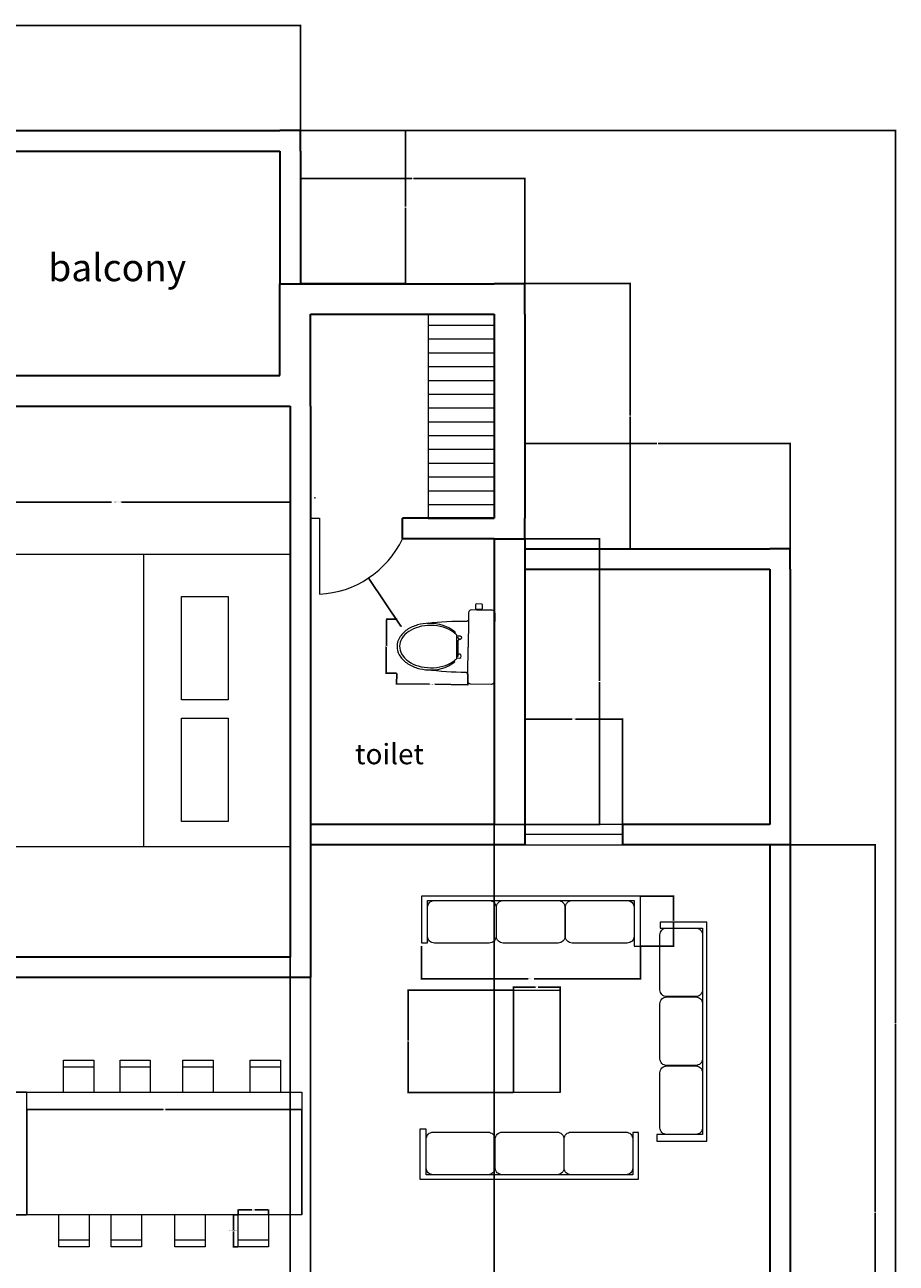
# Model space of a CAD drawing. Units: inches. Extents: x 177 to 785, y -381 to 206.
# Tile 5 of 5: x 529 to 785, y -158 to 206. Entities that reach past the tile are written whole.
import ezdxf

# ---------------------------------------------------------------- set-up
doc = ezdxf.new("R2010")
doc.units = ezdxf.units.IN
doc.header["$MEASUREMENT"] = 0
for name, color, linetype, lineweight in [('A-ANNO-DIMS', 2, 'Continuous', 18), ('A-AREA-IDEN', 7, 'Continuous', 20), ('A-DOOR', 4, 'Continuous', 18), ('A-FLOR-CASE', 9, 'Continuous', 20), ('A-FLOR-CASE-PATT', 9, 'Continuous', 13), ('A-FLOR-FIXT', 8, 'Continuous', 18), ('A-FURN', 2, 'Continuous', 18), ('A-GLAZ', 4, 'Continuous', 18), ('A-WALL', 7, 'Continuous', 35), ('WC-Detail_dwgmodels.com', 9, 'Continuous', 13), ('WC-Outline_dwgmodels.com', 8, 'Continuous', 18)]:
    doc.layers.add(name, color=color, linetype=linetype, lineweight=lineweight)
doc.styles.get("Standard").update_dxf_attribs({"font": 'arial.ttf'})
doc.dimstyles.get("Standard").update_dxf_attribs({"dimtxt": 0.18, "dimasz": 0.18, "dimexe": 0.18, "dimexo": 0.0625, "dimgap": 0.09, "dimtad": 0, "dimtih": 1, "dimtoh": 1, "dimdec": 4, "dimzin": 0, "dimdsep": 46, "dimtxsty": 'Standard', "dimcen": 0.09, "dimadec": 0, "dimazin": 0, "dimtfac": 1, "dimtdec": 4, "dimtofl": 0, "dimtmove": 0, "dimatfit": 3, "dimfxl": 1, "dimtolj": 1, "dimtzin": 0, "dimarcsym": 0})

# ---------------------------------------------------------------- blocks, each defined once
blk = doc.blocks.new('BED-DOUBLE')
blk.add_line((58.96, 86.04), (58.96, 0))
for points in [[(0, 86.04), (102.05, 86.04), (102.05, 0), (0, 0)], [(70.1, 73.56), (83.84, 73.56), (83.84, 43.2), (70.1, 43.2)], [(70.1, 37.79), (83.84, 37.79), (83.84, 7.42), (70.1, 7.42)]]:
    blk.add_lwpolyline(points, close=True)
blk = doc.blocks.new('SOFA-3-SEAT')
for p, q in [((64.37, 14.65), (0, 14.65)), ((0, 14.65), (0, 0.95)), ((64.37, 0), (64.37, 14.65)), ((1.74, 11.38), (1.74, 13.38)), ((1.74, 13.38), (62.42, 13.38)), ((62.42, 13.38), (62.42, 0)), ((0, 0.95), (1.74, 0.95)), ((1.74, 0.95), (1.74, 2.86)), ((62.42, 0), (64.37, 0))]:
    blk.add_line(p, q)
for points in [[(3.74, 13.38), (19.89, 13.38, -0.414214), (21.89, 11.38), (21.89, 2.86, -0.414214), (19.89, 0.86), (3.74, 0.86, -0.414214), (1.74, 2.86), (1.74, 11.38, -0.414214)], [(23.98, 13.38), (40.13, 13.38, -0.414214), (42.13, 11.38), (42.13, 2.86, -0.414214), (40.13, 0.86), (23.98, 0.86, -0.414214), (21.98, 2.86), (21.98, 11.38, -0.414214)], [(44.27, 13.38), (60.42, 13.38, -0.414214), (62.42, 11.38), (62.42, 2.86, -0.414214), (60.42, 0.86), (44.27, 0.86, -0.414214), (42.27, 2.86), (42.27, 11.38, -0.414214)]]:
    blk.add_lwpolyline(points, format="xyb", close=True)
blk = doc.blocks.new('CHAIR-DINING')
for p, q in [((0, 9.42), (8.88, 9.42)), ((0, 7.42), (0, 9.42)), ((0, 0), (0, 7.42)), ((0, 7.42), (8.88, 7.42)), ((8.88, 9.42), (8.88, 7.42)), ((8.88, 7.42), (8.88, 0))]:
    blk.add_line(p, q)
blk = doc.blocks.new('WC-PAN-AND-SEAT')
for points in [[(0, 20.91, -0.279901), (0.43, 20.4, 0.030761), (1.12, 8.8, 16.522544)], [(15.88, 20.91, 0.279901), (15.45, 20.4, -0.030761), (14.76, 8.8, -16.522544)], [(1.08, 9.29, -0.186192), (3.55, 17.08), (3.86, 16.84)], [(1.72, 9.92, 0.068564), (2.22, 6.28, 0.080689), (3.54, 3.43, 0.107047), (5.7, 1.38, 0.137952), (7.94, 0.75, 0.137952), (10.18, 1.38, 0.107047), (12.34, 3.43, 0.080689), (13.66, 6.28, 0.068564), (14.16, 9.92, 0.068564), (13.66, 13.57, 0.080689), (12.34, 16.41, 0.049741), (11.45, 17.48, 0.137952)], [(4.44, 17.48, 0.049741), (3.54, 16.41, 0.080689), (2.22, 13.57, 0.068564), (1.72, 9.92, 0.068564)], [(14.76, 8.8, 0.197511), (12.33, 17.08), (12.02, 16.84)], [(1.07, 9.29, 0.059006), (1.61, 5.99, 0.081908), (3.07, 2.91, 0.106902), (5.45, 0.69, 0.135271), (7.94, 0, 0.135271)], [(1.12, 8.8, -0.010918), (1.08, 9.29)], [(7.94, 0, 0.135271), (10.44, 0.69, 0.106902), (12.81, 2.91, 0.081908), (14.28, 5.99, 0.059006), (14.82, 9.29, 0.070136)]]:
    blk.add_lwpolyline(points, format="xyb")
blk.add_lwpolyline([(4.44, 17.48), (11.45, 17.48)])
blk = doc.blocks.new('*D9')
at = {"layer": 'A-ANNO-DIMS', "color": 0, "lineweight": -2, "transparency": 16777216}
for p, q in [((592, -143.94), (590.47, -143.94)), ((590.65, -144.12), (590.65, -148.47)), ((590.65, -153.18), (590.65, -148.83)), ((592, -153.36), (590.47, -153.36))]:
    blk.add_line(p, q, dxfattribs=at)
at = {"layer": 'A-ANNO-DIMS', "color": 0, "transparency": 16777216}
for points in [[(590.62, -144.12), (590.68, -144.12), (590.65, -143.94)], [(590.62, -153.18), (590.68, -153.18), (590.65, -153.36)]]:
    blk.add_solid(points, dxfattribs=at)
at = {"layer": 'Defpoints', "color": 0, "transparency": 16777216}
for p in [(592.07, -143.94), (590.65, -153.36), (592.07, -153.36)]:
    blk.add_point(p, dxfattribs=at)
at = {"layer": 'A-ANNO-DIMS', "color": 0, "transparency": 16777216, "insert": (590.65, -148.65), "char_height": 0.18, "attachment_point": 5}
blk.add_mtext('\\A1;DINING CHAIR 9 TYP.', dxfattribs=at)
blk = doc.blocks.new('*D10')
at = {"layer": 'A-ANNO-DIMS', "color": 0, "lineweight": -2, "transparency": 16777216}
for p, q in [((592.07, -143.88), (592.07, -142.34)), ((592.25, -142.52), (596.05, -142.52)), ((600.77, -142.52), (596.96, -142.52)), ((600.95, -143.88), (600.95, -142.34))]:
    blk.add_line(p, q, dxfattribs=at)
at = {"layer": 'A-ANNO-DIMS', "color": 0, "transparency": 16777216}
for points in [[(592.25, -142.49), (592.25, -142.55), (592.07, -142.52)], [(600.77, -142.49), (600.77, -142.55), (600.95, -142.52)]]:
    blk.add_solid(points, dxfattribs=at)
at = {"layer": 'Defpoints', "color": 0, "transparency": 16777216}
for p in [(592.07, -142.52), (592.07, -143.94), (600.95, -143.94)]:
    blk.add_point(p, dxfattribs=at)
at = {"layer": 'A-ANNO-DIMS', "color": 0, "transparency": 16777216, "insert": (596.51, -142.52), "char_height": 0.18, "attachment_point": 5}
blk.add_mtext('\\A1;9 TYP.', dxfattribs=at)
blk = doc.blocks.new('*D13')
at = {"layer": 'A-ANNO-DIMS', "color": 0, "lineweight": -2, "transparency": 16777216}
for p, q in [((505.28, 50.4), (505.28, 65.83)), ((505.46, 65.65), (554.86, 65.65)), ((607.15, 65.65), (557.74, 65.65)), ((607.33, 50.4), (607.33, 65.83))]:
    blk.add_line(p, q, dxfattribs=at)
at = {"layer": 'A-ANNO-DIMS', "color": 0, "transparency": 16777216}
for points in [[(505.46, 65.68), (505.46, 65.62), (505.28, 65.65)], [(607.15, 65.68), (607.15, 65.62), (607.33, 65.65)]]:
    blk.add_solid(points, dxfattribs=at)
at = {"layer": 'Defpoints', "color": 0, "transparency": 16777216}
for p in [(607.33, 65.65), (505.28, 50.34), (607.33, 50.34)]:
    blk.add_point(p, dxfattribs=at)
at = {"layer": 'A-ANNO-DIMS', "color": 0, "transparency": 16777216, "insert": (556.3, 65.65), "char_height": 0.18, "attachment_point": 5}
blk.add_mtext('\\A1;DOUBLE BED 102 TYP.', dxfattribs=at)
blk = doc.blocks.new('*D15')
at = {"layer": 'A-ANNO-DIMS', "color": 0, "lineweight": -2, "transparency": 16777216}
for p, q in [((645.99, -64.97), (645.99, -74.74)), ((710.36, -64.97), (710.36, -74.74)), ((646.17, -74.56), (677.27, -74.56)), ((710.18, -74.56), (679.08, -74.56))]:
    blk.add_line(p, q, dxfattribs=at)
at = {"layer": 'A-ANNO-DIMS', "color": 0, "transparency": 16777216}
for points in [[(646.17, -74.53), (646.17, -74.59), (645.99, -74.56)], [(710.18, -74.53), (710.18, -74.59), (710.36, -74.56)]]:
    blk.add_solid(points, dxfattribs=at)
at = {"layer": 'Defpoints', "color": 0, "transparency": 16777216}
for p in [(645.99, -64.91), (710.36, -64.91), (710.36, -74.56)]:
    blk.add_point(p, dxfattribs=at)
at = {"layer": 'A-ANNO-DIMS', "color": 0, "transparency": 16777216, "insert": (678.17, -74.56), "char_height": 0.18, "attachment_point": 5}
blk.add_mtext('\\A1;SOFA 64 TYP.', dxfattribs=at)
blk = doc.blocks.new('*D16')
at = {"layer": 'A-ANNO-DIMS', "color": 0, "lineweight": -2, "transparency": 16777216}
for p, q in [((710.42, -50.26), (720.19, -50.26)), ((720.01, -50.44), (720.01, -57.4)), ((720.01, -64.73), (720.01, -57.77)), ((710.42, -64.91), (720.19, -64.91))]:
    blk.add_line(p, q, dxfattribs=at)
at = {"layer": 'A-ANNO-DIMS', "color": 0, "transparency": 16777216}
for points in [[(719.98, -50.44), (720.04, -50.44), (720.01, -50.26)], [(719.98, -64.73), (720.04, -64.73), (720.01, -64.91)]]:
    blk.add_solid(points, dxfattribs=at)
at = {"layer": 'Defpoints', "color": 0, "transparency": 16777216}
for p in [(710.36, -50.26), (720.01, -50.26), (710.36, -64.91)]:
    blk.add_point(p, dxfattribs=at)
at = {"layer": 'A-ANNO-DIMS', "color": 0, "transparency": 16777216, "insert": (720.01, -57.58), "char_height": 0.18, "attachment_point": 5}
blk.add_mtext('\\A1;15 TYP.', dxfattribs=at)
blk = doc.blocks.new('*D17')
at = {"layer": 'A-ANNO-DIMS', "color": 0, "lineweight": -2, "transparency": 16777216}
for p, q in [((638.65, 15.24), (638.62, 11.99)), ((659.56, 15.01), (659.52, 11.76)), ((638.8, 12.17), (648.29, 12.06)), ((659.34, 11.94), (649.85, 12.05))]:
    blk.add_line(p, q, dxfattribs=at)
at = {"layer": 'A-ANNO-DIMS', "color": 0, "transparency": 16777216}
for points in [[(638.8, 12.2), (638.8, 12.14), (638.62, 12.17)], [(659.34, 11.97), (659.34, 11.91), (659.52, 11.94)]]:
    blk.add_solid(points, dxfattribs=at)
at = {"layer": 'Defpoints', "color": 0, "transparency": 16777216}
for p in [(638.65, 15.31), (659.56, 15.07), (659.52, 11.94)]:
    blk.add_point(p, dxfattribs=at)
at = {"layer": 'A-ANNO-DIMS', "color": 0, "transparency": 16777216, "insert": (649.07, 12.05), "char_height": 0.18, "attachment_point": 5}
blk.add_mtext('\\A1;WC 21 TYP.', dxfattribs=at)
blk = doc.blocks.new('*D18')
at = {"layer": 'A-ANNO-DIMS', "color": 0, "lineweight": -2, "transparency": 16777216}
for p, q in [((638.77, 31.19), (635.51, 31.22)), ((635.69, 31.04), (635.61, 23.46)), ((635.52, 15.52), (635.6, 23.1)), ((638.59, 15.31), (635.34, 15.34))]:
    blk.add_line(p, q, dxfattribs=at)
at = {"layer": 'A-ANNO-DIMS', "color": 0, "transparency": 16777216}
for points in [[(635.66, 31.04), (635.72, 31.04), (635.69, 31.22)], [(635.49, 15.52), (635.55, 15.52), (635.52, 15.34)]]:
    blk.add_solid(points, dxfattribs=at)
at = {"layer": 'Defpoints', "color": 0, "transparency": 16777216}
for p in [(638.83, 31.19), (635.52, 15.34), (638.65, 15.31)]:
    blk.add_point(p, dxfattribs=at)
at = {"layer": 'A-ANNO-DIMS', "color": 0, "transparency": 16777216, "insert": (635.61, 23.28), "char_height": 0.18, "attachment_point": 5}
blk.add_mtext('\\A1;16 TYP.', dxfattribs=at)
blk = doc.blocks.new('*D24')
at = {"layer": 'A-ANNO-DIMS', "color": 0, "lineweight": -2, "transparency": 16777216}
for p, q in [((610.39, 174.86), (785.46, 174.86)), ((785.28, 174.68), (785.28, -87.46)), ((785.28, -349.96), (785.28, -87.82)), ((537.67, -350.14), (785.46, -350.14))]:
    blk.add_line(p, q, dxfattribs=at)
at = {"layer": 'A-ANNO-DIMS', "color": 0, "transparency": 16777216}
for points in [[(785.25, 174.68), (785.31, 174.68), (785.28, 174.86)], [(785.25, -349.96), (785.31, -349.96), (785.28, -350.14)]]:
    blk.add_solid(points, dxfattribs=at)
at = {"layer": 'Defpoints', "color": 0, "transparency": 16777216}
for p in [(610.33, 174.86), (537.61, -350.14), (785.28, -350.14)]:
    blk.add_point(p, dxfattribs=at)
at = {"layer": 'A-ANNO-DIMS', "color": 0, "transparency": 16777216, "insert": (785.28, -87.64), "char_height": 0.18, "attachment_point": 5}
blk.add_mtext('\\A1;525', dxfattribs=at)
blk = doc.blocks.new('*D27')
at = {"layer": 'A-ANNO-DIMS', "color": 0, "lineweight": -2, "transparency": 16777216}
for p, q in [((355.33, 174.92), (355.33, 205.99)), ((355.51, 205.81), (482.54, 205.81)), ((610.15, 205.81), (483.12, 205.81)), ((610.33, 174.92), (610.33, 205.99))]:
    blk.add_line(p, q, dxfattribs=at)
at = {"layer": 'A-ANNO-DIMS', "color": 0, "transparency": 16777216}
for points in [[(355.51, 205.84), (355.51, 205.78), (355.33, 205.81)], [(610.15, 205.84), (610.15, 205.78), (610.33, 205.81)]]:
    blk.add_solid(points, dxfattribs=at)
at = {"layer": 'Defpoints', "color": 0, "transparency": 16777216}
for p in [(610.33, 205.81), (355.33, 174.86), (610.33, 174.86)]:
    blk.add_point(p, dxfattribs=at)
at = {"layer": 'A-ANNO-DIMS', "color": 0, "transparency": 16777216, "insert": (482.83, 205.81), "char_height": 0.18, "attachment_point": 5}
blk.add_mtext('\\A1;255', dxfattribs=at)
blk = doc.blocks.new('*D28')
at = {"layer": 'A-ANNO-DIMS', "color": 0, "lineweight": -2, "transparency": 16777216}
for p, q in [((610.33, 129.92), (610.33, 160.99)), ((610.51, 160.81), (643.11, 160.81)), ((676.15, 160.81), (643.55, 160.81)), ((676.33, 129.92), (676.33, 160.99))]:
    blk.add_line(p, q, dxfattribs=at)
at = {"layer": 'A-ANNO-DIMS', "color": 0, "transparency": 16777216}
for points in [[(610.51, 160.84), (610.51, 160.78), (610.33, 160.81)], [(676.15, 160.84), (676.15, 160.78), (676.33, 160.81)]]:
    blk.add_solid(points, dxfattribs=at)
at = {"layer": 'Defpoints', "color": 0, "transparency": 16777216}
for p in [(676.33, 160.81), (610.33, 129.86), (676.33, 129.86)]:
    blk.add_point(p, dxfattribs=at)
at = {"layer": 'A-ANNO-DIMS', "color": 0, "transparency": 16777216, "insert": (643.33, 160.81), "char_height": 0.18, "attachment_point": 5}
blk.add_mtext('\\A1;66', dxfattribs=at)
blk = doc.blocks.new('*D29')
at = {"layer": 'A-ANNO-DIMS', "color": 0, "lineweight": -2, "transparency": 16777216}
for p, q in [((676.33, 51.95), (676.33, 83.01)), ((676.51, 82.83), (715.11, 82.83)), ((754.15, 82.83), (715.55, 82.83)), ((754.33, 51.95), (754.33, 83.01))]:
    blk.add_line(p, q, dxfattribs=at)
at = {"layer": 'A-ANNO-DIMS', "color": 0, "transparency": 16777216}
for points in [[(676.51, 82.86), (676.51, 82.8), (676.33, 82.83)], [(754.15, 82.86), (754.15, 82.8), (754.33, 82.83)]]:
    blk.add_solid(points, dxfattribs=at)
at = {"layer": 'Defpoints', "color": 0, "transparency": 16777216}
for p in [(754.33, 82.83), (676.33, 51.88), (754.33, 51.88)]:
    blk.add_point(p, dxfattribs=at)
at = {"layer": 'A-ANNO-DIMS', "color": 0, "transparency": 16777216, "insert": (715.33, 82.83), "char_height": 0.18, "attachment_point": 5}
blk.add_mtext('\\A1;78', dxfattribs=at)
blk = doc.blocks.new('*D30')
at = {"layer": 'A-ANNO-DIMS', "color": 0, "lineweight": -2, "transparency": 16777216}
for p, q in [((610.39, 174.86), (641.46, 174.86)), ((641.28, 174.68), (641.28, 152.54)), ((641.28, 130.04), (641.28, 152.18)), ((610.39, 129.86), (641.46, 129.86))]:
    blk.add_line(p, q, dxfattribs=at)
at = {"layer": 'A-ANNO-DIMS', "color": 0, "transparency": 16777216}
for points in [[(641.25, 174.68), (641.31, 174.68), (641.28, 174.86)], [(641.25, 130.04), (641.31, 130.04), (641.28, 129.86)]]:
    blk.add_solid(points, dxfattribs=at)
at = {"layer": 'Defpoints', "color": 0, "transparency": 16777216}
for p in [(610.33, 174.86), (610.33, 129.86), (641.28, 129.86)]:
    blk.add_point(p, dxfattribs=at)
at = {"layer": 'A-ANNO-DIMS', "color": 0, "transparency": 16777216, "insert": (641.28, 152.36), "char_height": 0.18, "attachment_point": 5}
blk.add_mtext('\\A1;45', dxfattribs=at)
blk = doc.blocks.new('*D33')
at = {"layer": 'A-ANNO-DIMS', "color": 0, "lineweight": -2, "transparency": 16777216}
for p, q in [((607.33, -68.2), (607.33, -381.27)), ((439.33, -74.2), (439.33, -381.27)), ((439.51, -381.09), (523.05, -381.09)), ((607.15, -381.09), (523.61, -381.09))]:
    blk.add_line(p, q, dxfattribs=at)
at = {"layer": 'A-ANNO-DIMS', "color": 0, "transparency": 16777216}
for points in [[(439.51, -381.06), (439.51, -381.12), (439.33, -381.09)], [(607.15, -381.06), (607.15, -381.12), (607.33, -381.09)]]:
    blk.add_solid(points, dxfattribs=at)
at = {"layer": 'Defpoints', "color": 0, "transparency": 16777216}
for p in [(607.33, -68.14), (439.33, -74.14), (607.33, -381.09)]:
    blk.add_point(p, dxfattribs=at)
at = {"layer": 'A-ANNO-DIMS', "color": 0, "transparency": 16777216, "insert": (523.33, -381.09), "char_height": 0.18, "attachment_point": 5}
blk.add_mtext('\\A1;168', dxfattribs=at)
blk = doc.blocks.new('*D38')
at = {"layer": 'A-ANNO-DIMS', "color": 0, "lineweight": -2, "transparency": 16777216}
for p, q in [((676.39, 129.86), (707.46, 129.86)), ((707.28, 129.68), (707.28, 91.05)), ((707.28, 52.06), (707.28, 90.69)), ((676.39, 51.88), (707.46, 51.88))]:
    blk.add_line(p, q, dxfattribs=at)
at = {"layer": 'A-ANNO-DIMS', "color": 0, "transparency": 16777216}
for points in [[(707.25, 129.68), (707.31, 129.68), (707.28, 129.86)], [(707.25, 52.06), (707.31, 52.06), (707.28, 51.88)]]:
    blk.add_solid(points, dxfattribs=at)
at = {"layer": 'Defpoints', "color": 0, "transparency": 16777216}
for p in [(676.33, 129.86), (676.33, 51.88), (707.28, 51.88)]:
    blk.add_point(p, dxfattribs=at)
at = {"layer": 'A-ANNO-DIMS', "color": 0, "transparency": 16777216, "insert": (707.28, 90.87), "char_height": 0.18, "attachment_point": 5}
blk.add_mtext('\\A1;77.98', dxfattribs=at)
blk = doc.blocks.new('*D39')
at = {"layer": 'A-ANNO-DIMS', "color": 0, "lineweight": -2, "transparency": 16777216}
for p, q in [((667.39, 54.86), (698.46, 54.86)), ((698.28, 54.68), (698.28, 13.04)), ((698.28, -28.96), (698.28, 12.68)), ((667.39, -29.14), (698.46, -29.14))]:
    blk.add_line(p, q, dxfattribs=at)
at = {"layer": 'A-ANNO-DIMS', "color": 0, "transparency": 16777216}
for points in [[(698.25, 54.68), (698.31, 54.68), (698.28, 54.86)], [(698.25, -28.96), (698.31, -28.96), (698.28, -29.14)]]:
    blk.add_solid(points, dxfattribs=at)
at = {"layer": 'Defpoints', "color": 0, "transparency": 16777216}
for p in [(667.33, 54.86), (667.33, -29.14), (698.28, -29.14)]:
    blk.add_point(p, dxfattribs=at)
at = {"layer": 'A-ANNO-DIMS', "color": 0, "transparency": 16777216, "insert": (698.28, 12.86), "char_height": 0.18, "attachment_point": 5}
blk.add_mtext('\\A1;84', dxfattribs=at)
blk = doc.blocks.new('*D40')
at = {"layer": 'A-ANNO-DIMS', "color": 0, "lineweight": -2, "transparency": 16777216}
for p, q in [((613.33, -29.2), (613.33, -381.27)), ((667.33, -29.2), (667.33, -381.27)), ((613.51, -381.09), (640.11, -381.09)), ((667.15, -381.09), (640.55, -381.09))]:
    blk.add_line(p, q, dxfattribs=at)
at = {"layer": 'A-ANNO-DIMS', "color": 0, "transparency": 16777216}
for points in [[(613.51, -381.06), (613.51, -381.12), (613.33, -381.09)], [(667.15, -381.06), (667.15, -381.12), (667.33, -381.09)]]:
    blk.add_solid(points, dxfattribs=at)
at = {"layer": 'Defpoints', "color": 0, "transparency": 16777216}
for p in [(613.33, -29.14), (667.33, -29.14), (667.33, -381.09)]:
    blk.add_point(p, dxfattribs=at)
at = {"layer": 'A-ANNO-DIMS', "color": 0, "transparency": 16777216, "insert": (640.33, -381.09), "char_height": 0.18, "attachment_point": 5}
blk.add_mtext('\\A1;54', dxfattribs=at)
blk = doc.blocks.new('*D53')
at = {"layer": 'A-ANNO-DIMS', "color": 0, "lineweight": -2, "transparency": 16777216}
for p, q in [((748.39, -35.14), (779.46, -35.14)), ((779.28, -35.32), (779.28, -142.96)), ((779.28, -250.96), (779.28, -143.32)), ((748.39, -251.14), (779.46, -251.14))]:
    blk.add_line(p, q, dxfattribs=at)
at = {"layer": 'A-ANNO-DIMS', "color": 0, "transparency": 16777216}
for points in [[(779.25, -35.32), (779.31, -35.32), (779.28, -35.14)], [(779.25, -250.96), (779.31, -250.96), (779.28, -251.14)]]:
    blk.add_solid(points, dxfattribs=at)
at = {"layer": 'Defpoints', "color": 0, "transparency": 16777216}
for p in [(748.33, -35.14), (748.33, -251.14), (779.28, -251.14)]:
    blk.add_point(p, dxfattribs=at)
at = {"layer": 'A-ANNO-DIMS', "color": 0, "transparency": 16777216, "insert": (779.28, -143.14), "char_height": 0.18, "attachment_point": 5}
blk.add_mtext('\\A1;216', dxfattribs=at)
blk = doc.blocks.new('*D66')
at = {"layer": 'A-ANNO-DIMS', "color": 0, "lineweight": -2, "transparency": 16777216}
for p, q in [((529.93, -143.88), (529.93, -112.81)), ((610.77, -143.88), (610.77, -112.81)), ((530.11, -112.99), (569.96, -112.99)), ((610.59, -112.99), (570.74, -112.99))]:
    blk.add_line(p, q, dxfattribs=at)
at = {"layer": 'A-ANNO-DIMS', "color": 0, "transparency": 16777216}
for points in [[(530.11, -112.96), (530.11, -113.02), (529.93, -112.99)], [(610.59, -112.96), (610.59, -113.02), (610.77, -112.99)]]:
    blk.add_solid(points, dxfattribs=at)
at = {"layer": 'Defpoints', "color": 0, "transparency": 16777216}
for p in [(610.77, -112.99), (529.93, -143.94), (610.77, -143.94)]:
    blk.add_point(p, dxfattribs=at)
at = {"layer": 'A-ANNO-DIMS', "color": 0, "transparency": 16777216, "insert": (570.35, -112.99), "char_height": 0.18, "attachment_point": 5}
blk.add_mtext('\\A1;80.84', dxfattribs=at)
blk = doc.blocks.new('*D67')
at = {"layer": 'A-ANNO-DIMS', "color": 0, "lineweight": -2, "transparency": 16777216}
for p, q in [((529.87, -107.85), (498.8, -107.85)), ((498.98, -108.03), (498.98, -125.71)), ((498.98, -143.76), (498.98, -126.07)), ((529.87, -143.94), (498.8, -143.94))]:
    blk.add_line(p, q, dxfattribs=at)
at = {"layer": 'A-ANNO-DIMS', "color": 0, "transparency": 16777216}
for points in [[(498.95, -108.03), (499.01, -108.03), (498.98, -107.85)], [(498.95, -143.76), (499.01, -143.76), (498.98, -143.94)]]:
    blk.add_solid(points, dxfattribs=at)
at = {"layer": 'Defpoints', "color": 0, "transparency": 16777216}
for p in [(498.98, -107.85), (529.93, -107.85), (529.93, -143.94)]:
    blk.add_point(p, dxfattribs=at)
at = {"layer": 'A-ANNO-DIMS', "color": 0, "transparency": 16777216, "insert": (498.98, -125.89), "char_height": 0.18, "attachment_point": 5}
blk.add_mtext('\\A1;36.09', dxfattribs=at)
blk = doc.blocks.new('*D68')
at = {"layer": 'A-ANNO-DIMS', "color": 0, "lineweight": -2, "transparency": 16777216}
for p, q in [((672.92, -77.88), (641.86, -77.88)), ((642.04, -78.06), (642.04, -92.73)), ((642.04, -107.76), (642.04, -93.09)), ((672.92, -107.94), (641.86, -107.94))]:
    blk.add_line(p, q, dxfattribs=at)
at = {"layer": 'A-ANNO-DIMS', "color": 0, "transparency": 16777216}
for points in [[(642.01, -78.06), (642.07, -78.06), (642.04, -77.88)], [(642.01, -107.76), (642.07, -107.76), (642.04, -107.94)]]:
    blk.add_solid(points, dxfattribs=at)
at = {"layer": 'Defpoints', "color": 0, "transparency": 16777216}
for p in [(642.04, -77.88), (672.99, -77.88), (672.99, -107.94)]:
    blk.add_point(p, dxfattribs=at)
at = {"layer": 'A-ANNO-DIMS', "color": 0, "transparency": 16777216, "insert": (642.04, -92.91), "char_height": 0.18, "attachment_point": 5}
blk.add_mtext('\\A1;30.067', dxfattribs=at)
blk = doc.blocks.new('*D69')
at = {"layer": 'A-ANNO-DIMS', "color": 0, "lineweight": -2, "transparency": 16777216}
for p, q in [((672.99, -107.88), (672.99, -76.81)), ((673.17, -76.99), (679.47, -76.99)), ((686.55, -76.99), (680.24, -76.99)), ((686.73, -107.88), (686.73, -76.81))]:
    blk.add_line(p, q, dxfattribs=at)
at = {"layer": 'A-ANNO-DIMS', "color": 0, "transparency": 16777216}
for points in [[(673.17, -76.96), (673.17, -77.02), (672.99, -76.99)], [(686.55, -76.96), (686.55, -77.02), (686.73, -76.99)]]:
    blk.add_solid(points, dxfattribs=at)
at = {"layer": 'Defpoints', "color": 0, "transparency": 16777216}
for p in [(686.73, -76.99), (672.99, -107.94), (686.73, -107.94)]:
    blk.add_point(p, dxfattribs=at)
at = {"layer": 'A-ANNO-DIMS', "color": 0, "transparency": 16777216, "insert": (679.86, -76.99), "char_height": 0.18, "attachment_point": 5}
blk.add_mtext('\\A1;13.74', dxfattribs=at)
blk = doc.blocks.new('*D70')
at = {"layer": 'A-ANNO-DIMS', "color": 0, "lineweight": -2, "transparency": 16777216}
for p, q in [((676.33, -29.08), (676.33, 1.99)), ((676.51, 1.81), (690.23, 1.81)), ((704.89, 1.81), (691.17, 1.81)), ((705.07, -29.08), (705.07, 1.99))]:
    blk.add_line(p, q, dxfattribs=at)
at = {"layer": 'A-ANNO-DIMS', "color": 0, "transparency": 16777216}
for points in [[(676.51, 1.84), (676.51, 1.78), (676.33, 1.81)], [(704.89, 1.84), (704.89, 1.78), (705.07, 1.81)]]:
    blk.add_solid(points, dxfattribs=at)
at = {"layer": 'Defpoints', "color": 0, "transparency": 16777216}
for p in [(705.07, 1.81), (676.33, -29.14), (705.07, -29.14)]:
    blk.add_point(p, dxfattribs=at)
at = {"layer": 'A-ANNO-DIMS', "color": 0, "transparency": 16777216, "insert": (690.7, 1.81), "char_height": 0.18, "attachment_point": 5}
blk.add_mtext('\\A1;28.743', dxfattribs=at)
blk = doc.blocks.new('*D80')
at = {"layer": 'A-ANNO-DIMS', "color": 0, "lineweight": -2, "transparency": 16777216}
for p, q in [((614.54, 66.92), (614.72, 66.92)), ((614.63, 66.83), (614.63, 67.01)), ((639.86, 29.15), (630.5, 43.16)), ((640.04, 29.15), (639.86, 29.15))]:
    blk.add_line(p, q, dxfattribs=at)
at = {"layer": 'A-ANNO-DIMS', "color": 0, "transparency": 16777216}
blk.add_solid([(630.52, 43.18), (630.47, 43.15), (630.4, 43.31)], dxfattribs=at)
at = {"layer": 'Defpoints', "color": 0, "transparency": 16777216}
for p in [(614.63, 66.92), (630.4, 43.31)]:
    blk.add_point(p, dxfattribs=at)
at = {"layer": 'A-ANNO-DIMS', "color": 0, "transparency": 16777216, "insert": (640.52, 29.15), "char_height": 0.18, "attachment_point": 5}
blk.add_mtext('\\A1;R28.39', dxfattribs=at)

msp = doc.modelspace()

# ---------------------------------------------------------------- hatches: boundary and pattern name
at = {"layer": 'A-FLOR-CASE-PATT'}
h = msp.add_hatch(dxfattribs=at)
h.set_pattern_fill('ANSI31', color=256, scale=32.4574, angle=-45, style=0)
h.paths.add_polyline_path([(647.8995, 60.8599), (667.3284, 60.8599), (667.3284, 120.8599), (647.8995, 120.8599)])

# ---------------------------------------------------------------- linework, layer by layer
at = {"layer": 'A-DOOR'}
for p, q in [((613.3284, 60.8599), (615.93, 60.8599)), ((615.93, 60.8599), (615.93, 38.5601)), ((615.93, 38.5601), (615.93, 38.5601))]:
    msp.add_line(p, q, dxfattribs=at)
msp.add_arc((614.6292, 66.9175), 28.3872, 272.626382, 334.864837, dxfattribs=at)
at = {"layer": 'A-FLOR-CASE'}
for p, q in [((647.8995, 120.8599), (647.8995, 60.8599)), ((667.3284, 60.7137), (647.8995, 60.7137))]:
    msp.add_line(p, q, dxfattribs=at)
at = {"layer": 'A-FURN'}
for points in [[(672.9862, -77.8763), (686.7262, -77.8763), (686.7262, -107.9431), (672.9862, -107.9431)], [(529.9305, -107.8451), (610.7686, -107.8451), (610.7686, -143.9375), (529.9305, -143.9375)]]:
    msp.add_lwpolyline(points, close=True, dxfattribs=at)
at = {"layer": 'A-GLAZ'}
msp.add_line((705.0718, -32.1401), (676.3284, -32.1401), dxfattribs=at)
msp.add_lwpolyline([(676.3284, -35.1401), (705.0718, -35.1401), (705.0718, -29.1401), (676.3284, -29.1401)], close=True, dxfattribs=at)
at = {"layer": 'A-WALL'}
for p, q in [((521.8284, 174.8599), (604.3284, 174.8599)), ((610.3284, 174.8599), (604.3284, 174.8599)), ((610.3284, 168.8599), (610.3284, 174.8599)), ((515.8284, 168.8599), (604.3284, 168.8599)), ((604.3284, 168.8599), (604.3284, 129.8599)), ((610.3284, 168.8599), (610.3284, 129.8599)), ((604.3284, 120.8599), (604.3284, 129.8599)), ((604.3284, 129.8599), (613.3284, 129.8599)), ((613.3284, 129.8599), (667.3284, 129.8599)), ((676.3284, 129.8599), (667.3284, 129.8599)), ((676.3284, 120.8599), (676.3284, 129.8599)), ((604.3284, 102.8599), (604.3284, 120.8599)), ((613.3284, 102.8599), (613.3284, 120.8599)), ((613.3284, 120.8599), (667.3284, 120.8599)), ((667.3284, 120.8599), (667.3284, 60.8599)), ((676.3284, 120.8599), (676.3284, 60.8599)), ((504.7052, 102.8599), (604.3284, 102.8599)), ((613.3284, 93.8599), (613.3284, 102.8599)), ((504.7052, 93.8599), (607.3284, 93.8599)), ((607.3284, 93.8599), (607.3284, -68.1401)), ((613.3284, 93.8599), (613.3284, -38.1401)), ((667.3284, 60.8599), (640.3284, 60.8599)), ((640.3284, 54.8599), (640.3284, 60.8599)), ((676.3284, 54.8599), (676.3284, 60.8599)), ((667.3284, 54.8599), (640.3284, 54.8599)), ((667.3284, 54.8599), (676.3284, 54.8599)), ((667.3284, 54.8599), (667.3284, -29.1401)), ((676.3284, 54.8599), (676.3284, -29.1401)), ((676.3284, 51.8829), (748.3284, 51.8829)), ((754.3284, 51.8829), (748.3284, 51.8829)), ((754.3284, 45.8829), (754.3284, 51.8829)), ((676.3284, 45.8829), (748.3284, 45.8829)), ((748.3284, 45.8829), (748.3284, -29.1401)), ((754.3284, 45.8829), (754.3284, -35.1401)), ((667.3284, -29.1401), (613.3284, -29.1401)), ((676.3284, -29.1401), (676.3284, -35.1401)), ((748.3284, -29.1401), (705.0718, -29.1401)), ((705.0718, -29.1401), (705.0718, -35.1401)), ((676.3284, -35.1401), (613.3284, -35.1401)), ((748.3284, -35.1401), (705.0718, -35.1401)), ((754.3284, -35.1401), (748.3284, -35.1401)), ((748.3284, -35.1401), (748.3284, -251.1401)), ((754.3284, -35.1401), (754.3284, -257.1401)), ((613.3284, -38.1401), (613.3284, -68.1401)), ((607.3284, -68.1401), (495.3305, -68.1401)), ((613.3284, -68.1401), (613.3284, -74.1401)), ((613.3284, -74.1401), (495.3305, -74.1401))]:
    msp.add_line(p, q, dxfattribs=at)
at = {"layer": 'WC-Detail_dwgmodels.com'}
for points in [[(662.2091, 34.1292), (663.4688, 34.1152, 0.41421356)], [(656.2509, 25.8481), (656.6053, 25.8442, -0.41421356), (656.7999, 25.6452), (656.7934, 25.0547, -0.41421356), (656.5944, 24.86), (656.2401, 24.8639)], [(656.2562, 26.3205), (657.2797, 26.3092, -0.78819772), (657.2675, 25.2069), (656.7951, 25.2121)], [(656.1839, 19.7855), (657.2074, 19.7742, 0.78819772), (657.2196, 20.8765), (656.7472, 20.8817)], [(656.1891, 20.2579), (656.5434, 20.254, 0.41421356), (656.7424, 20.4486), (656.749, 21.0392, 0.41421356), (656.5543, 21.2382), (656.2, 21.2421)]]:
    msp.add_lwpolyline(points, format="xyb", dxfattribs=at)
msp.add_lwpolyline([(656.6337, 24.8596), (656.5937, 21.2377)], dxfattribs=at)
at = {"layer": 'WC-Outline_dwgmodels.com'}
for points in [[(662.2064, 33.893), (660.5924, 33.9108, 0.41421356), (659.7565, 33.0932), (659.7329, 30.9563)], [(661.7899, 35.3937), (661.7791, 34.4095, 0.41421356), (662.0516, 34.1309), (662.2091, 34.1292, 0.41421356)], [(663.4688, 34.1152), (663.6263, 34.1135, 0.41421356), (663.9049, 34.386), (663.9158, 35.3702, 0.41421356), (663.6433, 35.6488), (662.0686, 35.6662, 0.41421356), (661.7899, 35.3937)], [(663.4662, 33.879), (662.2064, 33.893, 0.41421356)], [(667.4398, 22.9289), (667.5513, 33.007, 0.41421356), (666.7337, 33.8429), (663.4662, 33.879, 0.41421356)], [(667.4398, 22.9289), (667.3283, 12.8508, -0.41421356), (666.4924, 12.0332), (660.3511, 12.1011, -0.41421356), (659.5335, 12.937), (659.5572, 15.0739)]]:
    msp.add_lwpolyline(points, format="xyb", dxfattribs=at)
for points in [[(662.2091, 34.1292), (662.2064, 33.893)], [(663.4688, 34.1152), (663.4662, 33.879)], [(659.7329, 30.9563), (659.645, 23.0151)], [(659.5572, 15.0739), (659.645, 23.0151)]]:
    msp.add_lwpolyline(points, dxfattribs=at)

# ---------------------------------------------------------------- block references
at = {"layer": 'A-FLOR-FIXT', "rotation": 269.3661547031217}
msp.add_blockref('WC-PAN-AND-SEAT', (638.8287, 31.1876), dxfattribs=at)
at = {"layer": 'A-FURN'}
for name, p in [('BED-DOUBLE', (505.275, -35.706)), ('SOFA-3-SEAT', (645.989, -64.908)), ('CHAIR-DINING', (540.713, -107.845)), ('CHAIR-DINING', (557.3271, -107.845)), ('CHAIR-DINING', (575.7901, -107.845)), ('CHAIR-DINING', (595.6246, -107.845))]:
    msp.add_blockref(name, p, dxfattribs=at)
for name, p, rotation in [('SOFA-3-SEAT', (715.1633, -57.9063), 270), ('SOFA-3-SEAT', (709.7733, -118.7885), 180), ('CHAIR-DINING', (548.219, -143.9377), 180), ('CHAIR-DINING', (563.5976, -143.9377), 180), ('CHAIR-DINING', (582.3561, -143.9377), 180), ('CHAIR-DINING', (600.9457, -143.9377), 180)]:
    msp.add_blockref(name, p, dxfattribs=dict(at, rotation=rotation))

# ---------------------------------------------------------------- texts
at = {"layer": 'A-AREA-IDEN', "attachment_point": 1}
for s, heights, insert, char_height in [('balcony', [6.0982], (536.2502, 138.5889), 8), ('toilet', [0], (626.4171, -5.4534), 6)]:
    msp.add_mtext_dynamic_manual_height_columns(s, width=20.406791, gutter_width=1, heights=heights, dxfattribs=dict(at, insert=insert, char_height=char_height))

# ---------------------------------------------------------------- dimensions: what is measured, and where the dimension line sits
at = {"layer": 'A-ANNO-DIMS'}
for base, p1, p2, override, picture, middle in [((610.3284, 205.8099), (355.3284, 174.8599), (610.3284, 174.8599), {"dimdec": 0, "dimlfac": 1, "dimrnd": 0, "dimzin": 0, "dimdsep": 46, "dimlunit": 2}, '*D27', (482.8284, 205.8099)), ((676.3284, 160.8099), (610.3284, 129.8599), (676.3284, 129.8599), {"dimdec": 0, "dimlfac": 1, "dimrnd": 0, "dimzin": 0, "dimdsep": 46, "dimlunit": 2}, '*D28', (643.3284, 160.8099)), ((754.3284, 82.8329), (676.3284, 51.8829), (754.3284, 51.8829), {"dimdec": 0, "dimlfac": 1, "dimrnd": 0, "dimzin": 0, "dimdsep": 46, "dimlunit": 2}, '*D29', (715.3284, 82.8329)), ((705.0718, 1.8099), (676.3284, -29.1401), (705.0718, -29.1401), {"dimdec": 3, "dimlfac": 1, "dimrnd": 0, "dimzin": 0, "dimdsep": 46, "dimlunit": 2}, '*D70', (690.7001, 1.8099)), ((667.3284, -381.0901), (613.3284, -29.1401), (667.3284, -29.1401), {"dimdec": 0, "dimlfac": 1, "dimrnd": 0, "dimzin": 0, "dimdsep": 46, "dimlunit": 2}, '*D40', (640.3284, -381.0901)), ((607.3284, -381.0901), (439.3284, -74.1401), (607.3284, -68.1401), {"dimdec": 0, "dimlfac": 1, "dimrnd": 0, "dimzin": 0, "dimdsep": 46, "dimlunit": 2}, '*D33', (523.3284, -381.0901)), ((686.7262, -76.9931), (672.9862, -107.9431), (686.7262, -107.9431), {"dimdec": 2, "dimlfac": 1, "dimrnd": 0, "dimzin": 0, "dimdsep": 46, "dimlunit": 2}, '*D69', (679.8562, -76.9931)), ((610.7686, -112.9875), (529.9305, -143.9375), (610.7686, -143.9375), {"dimdec": 2, "dimlfac": 1, "dimrnd": 0, "dimzin": 0, "dimdsep": 46, "dimlunit": 2}, '*D66', (570.3496, -112.9875))]:
    dim = msp.add_linear_dim(base=base, p1=p1, p2=p2, dimstyle='Standard', override=override, dxfattribs=at)
    dim.commit()
    dim.dimension.update_dxf_attribs({"geometry": picture, "text_midpoint": middle})
for base, p1, p2, angle, override, picture, middle in [((785.2784, -350.1401), (610.3284, 174.8599), (537.6096, -350.1401), 90, {"dimdec": 0, "dimlfac": 1, "dimrnd": 0, "dimzin": 0, "dimdsep": 46, "dimlunit": 2}, '*D24', (785.2784, -87.6401)), ((641.2784, 129.8599), (610.3284, 174.8599), (610.3284, 129.8599), 270, {"dimdec": 0, "dimlfac": 1, "dimrnd": 0, "dimzin": 0, "dimdsep": 46, "dimlunit": 2}, '*D30', (641.2784, 152.3599)), ((707.2784, 51.8829), (676.3284, 129.8599), (676.3284, 51.8829), 270, {"dimdec": 2, "dimlfac": 1, "dimrnd": 0, "dimzin": 0, "dimdsep": 46, "dimlunit": 2}, '*D38', (707.2784, 90.8714)), ((698.2784, -29.1401), (667.3284, 54.8599), (667.3284, -29.1401), 270, {"dimdec": 0, "dimlfac": 1, "dimrnd": 0, "dimzin": 0, "dimdsep": 46, "dimlunit": 2}, '*D39', (698.2784, 12.8599)), ((779.2784, -251.1401), (748.3284, -35.1401), (748.3284, -251.1401), 270, {"dimdec": 0, "dimlfac": 1, "dimrnd": 0, "dimzin": 0, "dimdsep": 46, "dimlunit": 2}, '*D53', (779.2784, -143.1401)), ((642.0362, -77.8763), (672.9862, -107.9431), (672.9862, -77.8763), 90, {"dimdec": 3, "dimlfac": 1, "dimrnd": 0, "dimzin": 0, "dimdsep": 46, "dimlunit": 2}, '*D68', (642.0362, -92.9097)), ((498.9805, -107.8451), (529.9305, -143.9375), (529.9305, -107.8451), 90, {"dimdec": 2, "dimlfac": 1, "dimrnd": 0, "dimzin": 0, "dimdsep": 46, "dimlunit": 2}, '*D67', (498.9805, -125.8913))]:
    dim = msp.add_linear_dim(base=base, p1=p1, p2=p2, angle=angle, dimstyle='Standard', override=override, dxfattribs=at)
    dim.commit()
    dim.dimension.update_dxf_attribs({"geometry": picture, "text_midpoint": middle})
for base, p1, p2, text, picture, middle in [((607.3284, 65.6459), (505.2755, 50.3379), (607.3284, 50.3379), 'DOUBLE BED <> TYP.', '*D13', (556.302, 65.6459)), ((710.3574, -74.5628), (645.9894, -64.9075), (710.3574, -64.9075), 'SOFA <> TYP.', '*D15', (678.1734, -74.5628))]:
    dim = msp.add_linear_dim(base=base, p1=p1, p2=p2, text=text, dimstyle='Standard', override={"dimdec": 0, "dimlfac": 1, "dimrnd": 0, "dimzin": 0, "dimdsep": 46, "dimlunit": 2}, dxfattribs=at)
    dim.commit()
    dim.dimension.update_dxf_attribs({"geometry": picture, "text_midpoint": middle})
dim = msp.add_radius_dim(center=(614.6292, 66.9175), mpoint=(630.3988, 43.3134), dimstyle='Standard', override={"dimdec": 2, "dimlfac": 1, "dimrnd": 0, "dimzin": 0, "dimdsep": 46, "dimlunit": 2}, dxfattribs=at)
dim.commit()
dim.dimension.update_dxf_attribs({"geometry": '*D80', "text_midpoint": (640.5205, 29.1509), "dimtype": 164})
for base, p1, p2, angle, text, picture, middle in [((635.5173, 15.3399), (638.8286, 31.1876), (638.6529, 15.3052), 269.366155, '<> TYP.', '*D18', (635.6051, 23.2811)), ((659.5225, 11.9383), (638.6529, 15.3052), (659.5572, 15.0739), 359.366155, 'WC <> TYP.', '*D17', (649.0703, 12.0539)), ((720.0126, -50.2616), (710.3574, -64.9075), (710.3574, -50.2616), 90, '<> TYP.', '*D16', (720.0126, -57.5846)), ((590.6524, -153.3609), (592.066, -143.9375), (592.066, -153.3609), 270, 'DINING CHAIR <> TYP.', '*D9', (590.6524, -148.6492)), ((592.066, -142.524), (600.9457, -143.9375), (592.066, -143.9375), 180, '<> TYP.', '*D10', (596.5058, -142.524))]:
    dim = msp.add_linear_dim(base=base, p1=p1, p2=p2, angle=angle, text=text, dimstyle='Standard', override={"dimdec": 0, "dimlfac": 1, "dimrnd": 0, "dimzin": 0, "dimdsep": 46, "dimlunit": 2}, dxfattribs=at)
    dim.commit()
    dim.dimension.update_dxf_attribs({"geometry": picture, "text_midpoint": middle})

doc.saveas('drawing.dxf')
